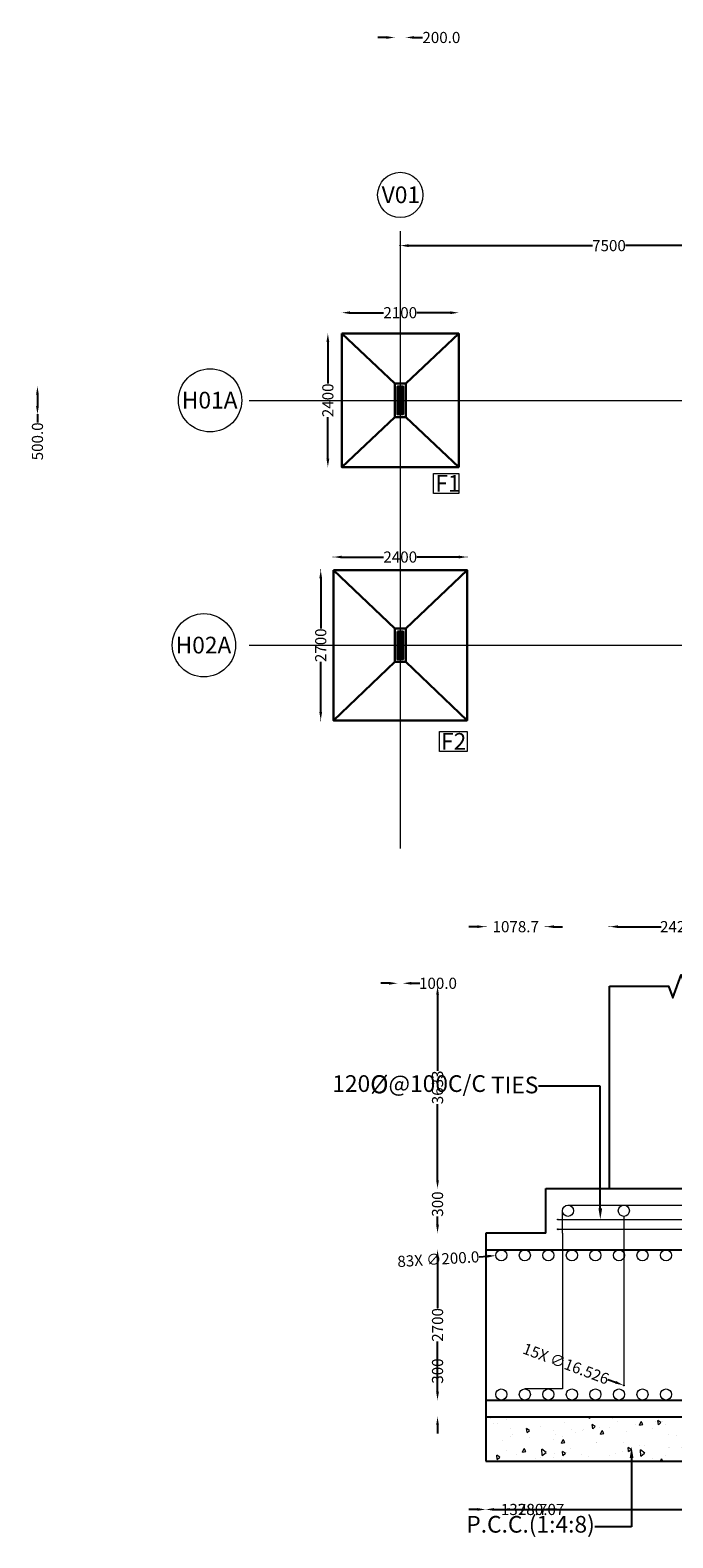
# Model space of a CAD drawing. Units: millimetres. Extents: x -30630 to 20484, y 3580 to 30715.
# Tile 1 of 4: x -30630 to -19082, y 3631 to 30715. Entities that reach past the tile are written whole.
import ezdxf
from ezdxf import colors
from ezdxf.entities.mleader import LeaderData, LeaderLine
from ezdxf.math import Vec2, Vec3

# ---------------------------------------------------------------- set-up
doc = ezdxf.new("R2010")
doc.units = ezdxf.units.MM
doc.header["$MEASUREMENT"] = 0
for name, color, linetype, lineweight in [('S-ANNO-DIMS', 2, 'Continuous', 18), ('S-ANNO-SYMB', 3, 'Continuous', 18), ('S-ANNO-TEXT', 7, 'Continuous', 18), ('S-CONC', 7, 'Continuous', 25), ('S-FNDN', 7, 'Continuous', 30), ('S-FNDN-PATT', 8, 'Continuous', 13), ('S-GRID', 1, 'Continuous', 18), ('S-GRID-IDEN', 7, 'Continuous', 18), ('S-REIN', 1, 'Continuous', 18)]:
    doc.layers.add(name, color=color, linetype=linetype, lineweight=lineweight)
doc.styles.get("Standard").update_dxf_attribs({"font": 'arial.ttf'})
doc.dimstyles.get("Standard").update_dxf_attribs({"dimtxt": 200, "dimasz": 150, "dimexe": 0.18, "dimexo": 0.0625, "dimgap": 0.09, "dimtad": 0, "dimdec": 0, "dimzin": 0, "dimdsep": 46, "dimtxsty": 'Standard', "dimcen": 0.09, "dimadec": 0, "dimazin": 0, "dimtfac": 1, "dimtdec": 0, "dimtofl": 0, "dimtmove": 0, "dimatfit": 3, "dimfxl": 1, "dimfxlon": 1, "dimtolj": 1, "dimtzin": 0, "dimarcsym": 0})

# ---------------------------------------------------------------- blocks, each defined once
blk = doc.blocks.new('*D1')
at = {"layer": 'Defpoints', "color": 0, "transparency": 16777216}
for p in [(-16480, 26844), (-23980, 25951), (-16480, 25951)]:
    blk.add_point(p, dxfattribs=at)
at = {"layer": 'S-ANNO-DIMS', "color": 0, "lineweight": -2, "transparency": 16777216}
for p, q in [((-23980, 26843), (-23980, 26844)), ((-23830, 26844), (-20528, 26844)), ((-16630, 26844), (-19933, 26844)), ((-16480, 26843), (-16480, 26844))]:
    blk.add_line(p, q, dxfattribs=at)
at = {"layer": 'S-ANNO-DIMS', "color": 0, "transparency": 16777216}
for points in [[(-23830, 26869), (-23830, 26819), (-23980, 26844)], [(-16630, 26869), (-16630, 26819), (-16480, 26844)]]:
    blk.add_solid(points, dxfattribs=at)
at = {"layer": 'S-ANNO-DIMS', "color": 0, "transparency": 16777216, "insert": (-20230, 26844), "char_height": 200, "attachment_point": 5}
blk.add_mtext('\\A1;7500', dxfattribs=at)
blk = doc.blocks.new('*D8')
at = {"layer": 'Defpoints', "color": 0, "transparency": 16777216}
for p in [(-22930, 25639), (-25030, 25265), (-22930, 25265)]:
    blk.add_point(p, dxfattribs=at)
at = {"layer": 'S-ANNO-DIMS', "color": 0, "lineweight": -2, "transparency": 16777216}
for p, q in [((-25030, 25638), (-25030, 25639)), ((-24880, 25639), (-24280, 25639)), ((-23080, 25639), (-23680, 25639)), ((-22930, 25638), (-22930, 25639))]:
    blk.add_line(p, q, dxfattribs=at)
at = {"layer": 'S-ANNO-DIMS', "color": 0, "transparency": 16777216}
for points in [[(-24880, 25664), (-24880, 25614), (-25030, 25639)], [(-23080, 25664), (-23080, 25614), (-22930, 25639)]]:
    blk.add_solid(points, dxfattribs=at)
at = {"layer": 'S-ANNO-DIMS', "color": 0, "transparency": 16777216, "insert": (-23980, 25639), "char_height": 200, "attachment_point": 5}
blk.add_mtext('\\A1;2100', dxfattribs=at)
blk = doc.blocks.new('*D9')
at = {"layer": 'Defpoints', "color": 0, "transparency": 16777216}
for p in [(-25030, 25265), (-25281, 22865), (-25030, 22865)]:
    blk.add_point(p, dxfattribs=at)
at = {"layer": 'S-ANNO-DIMS', "color": 0, "lineweight": -2, "transparency": 16777216}
for p, q in [((-25280, 25265), (-25281, 25265)), ((-25281, 25115), (-25281, 24365)), ((-25281, 23015), (-25281, 23765)), ((-25280, 22865), (-25281, 22865))]:
    blk.add_line(p, q, dxfattribs=at)
at = {"layer": 'S-ANNO-DIMS', "color": 0, "transparency": 16777216}
for points in [[(-25306, 25115), (-25256, 25115), (-25281, 25265)], [(-25306, 23015), (-25256, 23015), (-25281, 22865)]]:
    blk.add_solid(points, dxfattribs=at)
at = {"layer": 'S-ANNO-DIMS', "color": 0, "transparency": 16777216, "insert": (-25281, 24065), "char_height": 200, "attachment_point": 5, "rotation": 90}
blk.add_mtext('\\A1;2400', dxfattribs=at)
blk = doc.blocks.new('*D20')
at = {"layer": 'Defpoints', "color": 0, "transparency": 16777216}
for p in [(-25180, 21250), (-25180, 21015), (-22780, 21015)]:
    blk.add_point(p, dxfattribs=at)
at = {"layer": 'S-ANNO-DIMS', "color": 0, "lineweight": -2, "transparency": 16777216}
for p, q in [((-25180, 21249), (-25180, 21251)), ((-25030, 21250), (-24280, 21250)), ((-22930, 21250), (-23680, 21250)), ((-22780, 21249), (-22780, 21251))]:
    blk.add_line(p, q, dxfattribs=at)
at = {"layer": 'S-ANNO-DIMS', "color": 0, "transparency": 16777216}
for points in [[(-25030, 21275), (-25030, 21225), (-25180, 21250)], [(-22930, 21275), (-22930, 21225), (-22780, 21250)]]:
    blk.add_solid(points, dxfattribs=at)
at = {"layer": 'S-ANNO-DIMS', "color": 0, "transparency": 16777216, "insert": (-23980, 21250), "char_height": 200, "attachment_point": 5}
blk.add_mtext('\\A1;2400', dxfattribs=at)
blk = doc.blocks.new('*D21')
at = {"layer": 'Defpoints', "color": 0, "transparency": 16777216}
for p in [(-25180, 21015), (-25409, 18315), (-25180, 18315)]:
    blk.add_point(p, dxfattribs=at)
at = {"layer": 'S-ANNO-DIMS', "color": 0, "lineweight": -2, "transparency": 16777216}
for p, q in [((-25408, 21015), (-25410, 21015)), ((-25409, 20865), (-25409, 19965)), ((-25409, 18465), (-25409, 19365)), ((-25408, 18315), (-25410, 18315))]:
    blk.add_line(p, q, dxfattribs=at)
at = {"layer": 'S-ANNO-DIMS', "color": 0, "transparency": 16777216}
for points in [[(-25434, 20865), (-25384, 20865), (-25409, 21015)], [(-25434, 18465), (-25384, 18465), (-25409, 18315)]]:
    blk.add_solid(points, dxfattribs=at)
at = {"layer": 'S-ANNO-DIMS', "color": 0, "transparency": 16777216, "insert": (-25409, 19665), "char_height": 200, "attachment_point": 5, "rotation": 90}
blk.add_mtext('\\A1;2700', dxfattribs=at)
blk = doc.blocks.new('FOOTING-F1')
h = blk.add_hatch()
h.set_pattern_fill('ANSI31', color=256, scale=100)
h.set_pattern_definition([(45, (50626.339, 2179.544), (-8.8388348, 8.8388348), [])])
h.paths.add_polyline_path([(1100, 24315), (1000, 24315), (1000, 23815), (1100, 23815)])
for p, q in [((0, 25265), (950, 24365)), ((1150, 24365), (2100, 25265)), ((950, 23765), (0, 22865)), ((1150, 23765), (2100, 22865))]:
    blk.add_line(p, q)
for points in [[(0, 25265), (2100, 25265), (2100, 22865), (0, 22865)], [(950, 24365), (1150, 24365), (1150, 23765), (950, 23765)], [(1000, 24315), (1100, 24315), (1100, 23815), (1000, 23815)]]:
    blk.add_lwpolyline(points, close=True)
blk = doc.blocks.new('FOOTING-F2')
h = blk.add_hatch()
h.set_pattern_fill('ANSI31', color=256, scale=100)
h.set_pattern_definition([(45, (58801.161, 2265.705), (-8.8388348, 8.8388348), [])])
h.paths.add_polyline_path([(1250, 19915), (1150, 19915), (1150, 19415), (1250, 19415)])
for p, q in [((1100, 19965), (0, 21015)), ((1300, 19965), (2400, 21015)), ((1100, 19365), (0, 18315)), ((1300, 19365), (2400, 18315))]:
    blk.add_line(p, q)
for points in [[(0, 21015), (2400, 21015), (2400, 18315), (0, 18315)], [(1100, 19965), (1300, 19965), (1300, 19365), (1100, 19365)], [(1150, 19915), (1250, 19915), (1250, 19415), (1150, 19415)]]:
    blk.add_lwpolyline(points, close=True)
blk = doc.blocks.new('*D37')
at = {"layer": 'Defpoints', "color": 0, "transparency": 16777216}
for p in [(-23310, 6106), (-22445, 6106), (-22445, 5806)]:
    blk.add_point(p, dxfattribs=at)
at = {"layer": 'S-ANNO-DIMS', "color": 0, "lineweight": -2, "transparency": 16777216}
for p, q in [((-23310, 6256), (-23310, 6406)), ((-23309, 6106), (-23310, 6106)), ((-23309, 5806), (-23310, 5806)), ((-23310, 5656), (-23310, 5506))]:
    blk.add_line(p, q, dxfattribs=at)
at = {"layer": 'S-ANNO-DIMS', "color": 0, "transparency": 16777216}
for points in [[(-23335, 6256), (-23285, 6256), (-23310, 6106)], [(-23335, 5656), (-23285, 5656), (-23310, 5806)]]:
    blk.add_solid(points, dxfattribs=at)
at = {"layer": 'S-ANNO-DIMS', "color": 0, "transparency": 16777216, "insert": (-23310, 6627), "char_height": 200, "attachment_point": 5, "rotation": 90}
blk.add_mtext('\\A1;300', dxfattribs=at)
blk = doc.blocks.new('*D38')
at = {"layer": 'Defpoints', "color": 0, "transparency": 16777216}
for p in [(-23309.743439, 8806.371523), (-22444.743439, 8806.371523), (-22444.743439, 6106.371523)]:
    blk.add_point(p, dxfattribs=at)
at = {"layer": 'S-ANNO-DIMS', "color": 0, "lineweight": -2, "transparency": 16777216}
for p, q in [((-23308.743439, 8806.371523), (-23309.923439, 8806.371523)), ((-23309.743439, 8656.371523), (-23309.743439, 7756.461523)), ((-23309.743439, 6256.371523), (-23309.743439, 7156.281523)), ((-23308.743439, 6106.371523), (-23309.923439, 6106.371523))]:
    blk.add_line(p, q, dxfattribs=at)
at = {"layer": 'S-ANNO-DIMS', "color": 0, "transparency": 16777216}
for points in [[(-23334.743439, 8656.371523), (-23284.743439, 8656.371523), (-23309.743439, 8806.371523)], [(-23334.743439, 6256.371523), (-23284.743439, 6256.371523), (-23309.743439, 6106.371523)]]:
    blk.add_solid(points, dxfattribs=at)
at = {"layer": 'S-ANNO-DIMS', "color": 0, "transparency": 16777216, "insert": (-23309.743439, 7456.371523), "char_height": 200, "attachment_point": 5, "rotation": 90}
blk.add_mtext('\\A1;2700', dxfattribs=at)
blk = doc.blocks.new('*D39')
at = {"layer": 'Defpoints', "color": 0, "transparency": 16777216}
for p in [(-23310, 9106), (-22445, 9106), (-22445, 8806)]:
    blk.add_point(p, dxfattribs=at)
at = {"layer": 'S-ANNO-DIMS', "color": 0, "lineweight": -2, "transparency": 16777216}
for p, q in [((-23310, 9256), (-23310, 9406)), ((-23309, 9106), (-23310, 9106)), ((-23309, 8806), (-23310, 8806)), ((-23310, 8656), (-23310, 8506))]:
    blk.add_line(p, q, dxfattribs=at)
at = {"layer": 'S-ANNO-DIMS', "color": 0, "transparency": 16777216}
for points in [[(-23335, 9256), (-23285, 9256), (-23310, 9106)], [(-23335, 8656), (-23285, 8656), (-23310, 8806)]]:
    blk.add_solid(points, dxfattribs=at)
at = {"layer": 'S-ANNO-DIMS', "color": 0, "transparency": 16777216, "insert": (-23310, 9627), "char_height": 200, "attachment_point": 5, "rotation": 90}
blk.add_mtext('\\A1;300', dxfattribs=at)
blk = doc.blocks.new('*D40')
at = {"layer": 'Defpoints', "color": 0, "transparency": 16777216}
for p in [(-23310, 13539), (-12091, 13539), (-12091, 9906)]:
    blk.add_point(p, dxfattribs=at)
at = {"layer": 'S-ANNO-DIMS', "color": 0, "lineweight": -2, "transparency": 16777216}
for p, q in [((-23309, 13539), (-23310, 13539)), ((-23310, 13389), (-23310, 12021)), ((-23310, 10056), (-23310, 11424)), ((-23309, 9906), (-23310, 9906))]:
    blk.add_line(p, q, dxfattribs=at)
at = {"layer": 'S-ANNO-DIMS', "color": 0, "transparency": 16777216}
for points in [[(-23335, 13389), (-23285, 13389), (-23310, 13539)], [(-23335, 10056), (-23285, 10056), (-23310, 9906)]]:
    blk.add_solid(points, dxfattribs=at)
at = {"layer": 'S-ANNO-DIMS', "color": 0, "transparency": 16777216, "insert": (-23310, 11723), "char_height": 200, "attachment_point": 5, "rotation": 90}
blk.add_mtext('\\A1;3633', dxfattribs=at)
blk = doc.blocks.new('*D41')
at = {"layer": 'Defpoints', "color": 0, "transparency": 16777216}
for p in [(-21366, 14610), (-22445, 9106), (-21366, 9106)]:
    blk.add_point(p, dxfattribs=at)
at = {"layer": 'S-ANNO-DIMS', "color": 0, "lineweight": -2, "transparency": 16777216}
for p, q in [((-22595, 14610), (-22745, 14610)), ((-22445, 14609), (-22445, 14611)), ((-21366, 14609), (-21366, 14611)), ((-21216, 14610), (-21066, 14610))]:
    blk.add_line(p, q, dxfattribs=at)
at = {"layer": 'S-ANNO-DIMS', "color": 0, "transparency": 16777216}
for points in [[(-22595, 14635), (-22595, 14585), (-22445, 14610)], [(-21216, 14635), (-21216, 14585), (-21366, 14610)]]:
    blk.add_solid(points, dxfattribs=at)
at = {"layer": 'S-ANNO-DIMS', "color": 0, "transparency": 16777216, "insert": (-21905, 14610), "char_height": 200, "attachment_point": 5}
blk.add_mtext('\\A1;1078.7', dxfattribs=at)
blk = doc.blocks.new('*D43')
at = {"layer": 'Defpoints', "color": 0, "transparency": 16777216}
for p in [(-17798, 14610), (-20219, 13539), (-17798, 13539)]:
    blk.add_point(p, dxfattribs=at)
at = {"layer": 'S-ANNO-DIMS', "color": 0, "lineweight": -2, "transparency": 16777216}
for p, q in [((-20219, 14609), (-20219, 14611)), ((-20069, 14610), (-19290, 14610)), ((-17948, 14610), (-18727, 14610)), ((-17798, 14609), (-17798, 14611))]:
    blk.add_line(p, q, dxfattribs=at)
at = {"layer": 'S-ANNO-DIMS', "color": 0, "transparency": 16777216}
for points in [[(-20069, 14635), (-20069, 14585), (-20219, 14610)], [(-17948, 14635), (-17948, 14585), (-17798, 14610)]]:
    blk.add_solid(points, dxfattribs=at)
at = {"layer": 'S-ANNO-DIMS', "color": 0, "transparency": 16777216, "insert": (-19009, 14610), "char_height": 200, "attachment_point": 5}
blk.add_mtext('\\A1;2421', dxfattribs=at)
blk = doc.blocks.new('*D61')
at = {"layer": 'Defpoints', "color": 0, "transparency": 16777216}
for p in [(-19970, 6373), (-19955, 6368)]:
    blk.add_point(p, dxfattribs=at)
at = {"layer": 'S-ANNO-DIMS', "color": 0, "lineweight": -2, "transparency": 16777216}
for p, q in [((-20251, 6478), (-20111, 6426)), ((-19963, 6370), (-19963, 6371)), ((-19963, 6370), (-19962, 6370))]:
    blk.add_line(p, q, dxfattribs=at)
at = {"layer": 'S-ANNO-DIMS', "color": 0, "transparency": 16777216}
blk.add_solid([(-20102, 6449), (-20120, 6402), (-19970, 6373)], dxfattribs=at)
at = {"layer": 'S-ANNO-DIMS', "color": 0, "transparency": 16777216, "insert": (-21002, 6759), "char_height": 200, "attachment_point": 5, "rotation": 339.5143}
blk.add_mtext('\\A1;15X ∅16.526', dxfattribs=at)
blk = doc.blocks.new('*D64')
at = {"layer": 'Defpoints', "color": 0, "transparency": 16777216}
for p in [(-23880, 30583), (-24080, 24365), (-23880, 24365)]:
    blk.add_point(p, dxfattribs=at)
at = {"layer": 'S-ANNO-DIMS', "color": 0, "lineweight": -2, "transparency": 16777216}
for p, q in [((-24230, 30583), (-24380, 30583)), ((-24080, 30582), (-24080, 30584)), ((-23880, 30582), (-23880, 30584)), ((-23730, 30583), (-23580, 30583))]:
    blk.add_line(p, q, dxfattribs=at)
at = {"layer": 'S-ANNO-DIMS', "color": 0, "transparency": 16777216}
for points in [[(-24230, 30608), (-24230, 30558), (-24080, 30583)], [(-23730, 30608), (-23730, 30558), (-23880, 30583)]]:
    blk.add_solid(points, dxfattribs=at)
at = {"layer": 'S-ANNO-DIMS', "color": 0, "transparency": 16777216, "insert": (-23241, 30583), "char_height": 200, "attachment_point": 5}
blk.add_mtext('\\A1;200.0', dxfattribs=at)
blk = doc.blocks.new('*D65')
at = {"layer": 'Defpoints', "color": 0, "transparency": 16777216}
for p in [(-23880, 24365), (-23880, 23765), (19772, 23765)]:
    blk.add_point(p, dxfattribs=at)
at = {"layer": 'S-ANNO-DIMS', "color": 0, "lineweight": -2, "transparency": 16777216}
for p, q in [((19771, 24365), (19772, 24365)), ((19772, 24215), (19772, 23915)), ((19771, 23765), (19772, 23765)), ((19772, 23765), (19772, 23615))]:
    blk.add_line(p, q, dxfattribs=at)
at = {"layer": 'S-ANNO-DIMS', "color": 0, "transparency": 16777216}
for points in [[(19747, 24215), (19797, 24215), (19772, 24365)], [(19747, 23915), (19797, 23915), (19772, 23765)]]:
    blk.add_solid(points, dxfattribs=at)
at = {"layer": 'S-ANNO-DIMS', "color": 0, "transparency": 16777216, "insert": (19772, 23277), "char_height": 200, "attachment_point": 5, "rotation": 90}
blk.add_mtext('\\A1;600.0', dxfattribs=at)
blk = doc.blocks.new('*D66')
at = {"layer": 'Defpoints', "color": 0, "transparency": 16777216}
for p in [(-24030, 23815), (-23930, 23815), (-23930, 13593)]:
    blk.add_point(p, dxfattribs=at)
at = {"layer": 'S-ANNO-DIMS', "color": 0, "lineweight": -2, "transparency": 16777216}
for p, q in [((-24180, 13593), (-24330, 13593)), ((-24030, 13594), (-24030, 13593)), ((-23930, 13594), (-23930, 13593)), ((-23780, 13593), (-23630, 13593))]:
    blk.add_line(p, q, dxfattribs=at)
at = {"layer": 'S-ANNO-DIMS', "color": 0, "transparency": 16777216}
for points in [[(-24180, 13618), (-24180, 13568), (-24030, 13593)], [(-23780, 13618), (-23780, 13568), (-23930, 13593)]]:
    blk.add_solid(points, dxfattribs=at)
at = {"layer": 'S-ANNO-DIMS', "color": 0, "transparency": 16777216, "insert": (-23302, 13593), "char_height": 200, "attachment_point": 5}
blk.add_mtext('\\A1;100.0', dxfattribs=at)
blk = doc.blocks.new('*D67')
at = {"layer": 'Defpoints', "color": 0, "transparency": 16777216}
for p in [(-24030, 24315), (-30499, 23815), (-24030, 23815)]:
    blk.add_point(p, dxfattribs=at)
at = {"layer": 'S-ANNO-DIMS', "color": 0, "lineweight": -2, "transparency": 16777216}
for p, q in [((-30498, 24315), (-30499, 24315)), ((-30499, 24165), (-30499, 23965)), ((-30498, 23815), (-30499, 23815)), ((-30499, 23815), (-30499, 23665))]:
    blk.add_line(p, q, dxfattribs=at)
at = {"layer": 'S-ANNO-DIMS', "color": 0, "transparency": 16777216}
for points in [[(-30524, 24165), (-30474, 24165), (-30499, 24315)], [(-30524, 23965), (-30474, 23965), (-30499, 23815)]]:
    blk.add_solid(points, dxfattribs=at)
at = {"layer": 'S-ANNO-DIMS', "color": 0, "transparency": 16777216, "insert": (-30499, 23328), "char_height": 200, "attachment_point": 5, "rotation": 90}
blk.add_mtext('\\A1;500.0', dxfattribs=at)
blk = doc.blocks.new('*D68')
at = {"layer": 'Defpoints', "color": 0, "transparency": 16777216}
for p in [(-22445, 6106), (-7445, 6106), (-7445, 4141)]:
    blk.add_point(p, dxfattribs=at)
at = {"layer": 'S-ANNO-DIMS', "color": 0, "lineweight": -2, "transparency": 16777216}
for p, q in [((-22445, 4142), (-22445, 4141)), ((-22295, 4141), (-15428, 4141)), ((-7595, 4141), (-14462, 4141)), ((-7445, 4142), (-7445, 4141))]:
    blk.add_line(p, q, dxfattribs=at)
at = {"layer": 'S-ANNO-DIMS', "color": 0, "transparency": 16777216}
for points in [[(-22295, 4166), (-22295, 4116), (-22445, 4141)], [(-7595, 4166), (-7595, 4116), (-7445, 4141)]]:
    blk.add_solid(points, dxfattribs=at)
at = {"layer": 'S-ANNO-DIMS', "color": 0, "transparency": 16777216, "insert": (-14945, 4141), "char_height": 200, "attachment_point": 5}
blk.add_mtext('\\A1;15000.0', dxfattribs=at)
blk = doc.blocks.new('*D69')
at = {"layer": 'Defpoints', "color": 0, "transparency": 16777216}
for p in [(-22445, 6106), (-22165, 6206), (-22165, 4141)]:
    blk.add_point(p, dxfattribs=at)
at = {"layer": 'S-ANNO-DIMS', "color": 0, "lineweight": -2, "transparency": 16777216}
for p, q in [((-22595, 4141), (-22745, 4141)), ((-22445, 4142), (-22445, 4141)), ((-22165, 4142), (-22165, 4141)), ((-22015, 4141), (-21865, 4141))]:
    blk.add_line(p, q, dxfattribs=at)
at = {"layer": 'S-ANNO-DIMS', "color": 0, "transparency": 16777216}
for points in [[(-22595, 4166), (-22595, 4116), (-22445, 4141)], [(-22015, 4166), (-22015, 4116), (-22165, 4141)]]:
    blk.add_solid(points, dxfattribs=at)
at = {"layer": 'S-ANNO-DIMS', "color": 0, "transparency": 16777216, "insert": (-21448, 4141), "char_height": 200, "attachment_point": 5}
blk.add_mtext('\\A1;280.07', dxfattribs=at)
blk = doc.blocks.new('*D71')
at = {"layer": 'Defpoints', "color": 0, "transparency": 16777216}
for p in [(-21066, 6306), (-22445, 6106), (-21066, 4141)]:
    blk.add_point(p, dxfattribs=at)
at = {"layer": 'S-ANNO-DIMS', "color": 0, "lineweight": -2, "transparency": 16777216}
for p, q in [((-22445, 4142), (-22445, 4141)), ((-22295, 4141), (-22161, 4141)), ((-21216, 4141), (-21350, 4141)), ((-21066, 4142), (-21066, 4141))]:
    blk.add_line(p, q, dxfattribs=at)
at = {"layer": 'S-ANNO-DIMS', "color": 0, "transparency": 16777216}
for points in [[(-22295, 4166), (-22295, 4116), (-22445, 4141)], [(-21216, 4166), (-21216, 4116), (-21066, 4141)]]:
    blk.add_solid(points, dxfattribs=at)
at = {"layer": 'S-ANNO-DIMS', "color": 0, "transparency": 16777216, "insert": (-21755, 4141), "char_height": 200, "attachment_point": 5}
blk.add_mtext('\\A1;1378.7', dxfattribs=at)
blk = doc.blocks.new('*D80')
at = {"layer": 'Defpoints', "color": 0, "transparency": 16777216}
for p in [(-22264, 8700), (-22065, 8712)]:
    blk.add_point(p, dxfattribs=at)
at = {"layer": 'S-ANNO-DIMS', "color": 0, "lineweight": -2, "transparency": 16777216}
for p, q in [((-22564, 8682), (-22414, 8691)), ((-22165, 8706), (-22165, 8706)), ((-22165, 8706), (-22165, 8706))]:
    blk.add_line(p, q, dxfattribs=at)
at = {"layer": 'S-ANNO-DIMS', "color": 0, "transparency": 16777216}
blk.add_solid([(-22416, 8716), (-22413, 8666), (-22264, 8700)], dxfattribs=at)
at = {"layer": 'S-ANNO-DIMS', "color": 0, "transparency": 16777216, "insert": (-23296, 8638), "char_height": 200, "attachment_point": 5, "rotation": 3.4778}
blk.add_mtext('\\A1;83X ∅200.0', dxfattribs=at)

msp = doc.modelspace()

# ---------------------------------------------------------------- hatches: boundary and pattern name
at = {"layer": 'S-FNDN-PATT'}
h = msp.add_hatch(dxfattribs=at)
h.set_pattern_fill('AR-CONC', color=256, scale=100, angle=47)
h.set_pattern_definition([(97, (-6254.7, 5540.77), (535.064, 481.774), [75, -825]), (42, (-6254.7, 5540.8), (-644.747, 411.518), [60, -660]), (147.4514, (-6210.1, 5580.9), (-109.682, 893.292), [63.74, -701.142]), (93.184, (-6401, 5677.2), (848.91, 667.647), [112.5, -1237.5]), (143.636, (-6330.2, 5732.8), (-74.99, 1347.916), [95.61, -1051.714]), (38.184, (-6401, 5677.2), (-74.99, 1347.916), [90, -990]), (68, (-6296.2, 5716.2), (701.546, 161.965), [75, -825]), (13, (-6296.2, 5716.2), (-364.4, 672.5), [60, -660]), (118.4514, (-6237.74, 5729.7), (337.146, 834.465), [63.74, -701.142]), (84.5, (-6254.7, 5540.77), (-235.17, 235.9262), [0, -652, 0, -670, 0, -662.5]), (54.5, (-6254.7, 5540.77), (-109.0415, 461.385), [0, -382, 0, -637, 0, -252.5]), (14.5, (-6406.8, 5377.67), (380.5616, 375.0306), [0, -250, 0, -780, 0, -1035]), (4.5, (-6475, 5304.54), (324.52, 494.787), [0, -325, 0, -518, 0, -735])])
h.paths.add_polyline_path([(-7444.7434, 5006.3715), (-7444.7434, 5806.3715), (-22444.7434, 5806.3715), (-22444.7434, 5006.3715)])

# ---------------------------------------------------------------- linework, layer by layer
at = {"layer": 'S-ANNO-SYMB'}
for points in [[(-23380.1095, 22391.7904), (-23380.1095, 22753.0183), (-22930.0685, 22753.0183), (-22930.0685, 22391.7904)], [(-23277.1763, 17757.175), (-23277.1763, 18118.4029), (-22780.0685, 18118.4029), (-22780.0685, 17757.175)]]:
    msp.add_lwpolyline(points, close=True, dxfattribs=at)
at = {"layer": 'S-CONC'}
for p, q in [((-20219.1563, 9906.3715), (-20219.1563, 13539.302)), ((-21366.0811, 9106.3715), (-21366.0811, 9906.3715)), ((-21366.0811, 9906.3715), (-14944.7434, 9906.3715)), ((-22444.7434, 9106.3715), (-22444.7434, 5806.3715)), ((-21366.0811, 9106.3715), (-22444.7434, 9106.3715)), ((-22444.7434, 8806.3715), (-7444.7434, 8806.3715)), ((-22444.7434, 6106.3715), (-7444.7434, 6106.3715)), ((-22444.7434, 5806.3715), (-7444.7434, 5806.3715)), ((-22444.7434, 5806.3715), (-22444.7434, 5006.3715)), ((-22444.7434, 5006.3715), (-7444.7434, 5006.3715))]:
    msp.add_line(p, q, dxfattribs=at)
msp.add_lwpolyline([(-20219.3363, 13539.302), (-19158.6753, 13539.302), (-19083.6753, 13333.2412), (-18933.6753, 13745.3628), (-18858.6753, 13539.302), (-17798.0143, 13539.302)], dxfattribs=at)
at = {"layer": 'S-GRID'}
for p, q in [((-23980.0685, 27102.0571), (-23980.0685, 16015.6561)), ((-26695.8159, 24064.7195), (17349.3354, 24064.7195)), ((-26695.8159, 19664.7195), (17349.3354, 19664.7195))]:
    msp.add_line(p, q, dxfattribs=at)
at = {"layer": 'S-GRID-IDEN'}
for centre, radius in [((-23980.0685, 27753.8802), 407.0061), ((-27396.6824, 24064.7195), 568.051), ((-27508.1703, 19664.7195), 568.051)]:
    msp.add_circle(centre, radius, dxfattribs=at)
at = {"layer": 'S-REIN'}
for p, q in [((-21066.0811, 9106.3715), (-21066.0811, 9506.3715)), ((-20966.0811, 9606.3715), (-14944.7434, 9606.3715)), ((-21140.5094, 9349.192), (-8740.6319, 9349.192)), ((-19962.5248, 9406.3715), (-19962.5248, 6378.7119)), ((-21140.5094, 9174.6041), (-8740.6319, 9174.6041)), ((-21066.0811, 9106.3715), (-21066.0811, 6306.3715)), ((-21066.0811, 6306.3715), (-21741.8353, 6306.3715))]:
    msp.add_line(p, q, dxfattribs=at)
for centre, radius in [((-20966.0811, 9506.3715), 100), ((-19962.5248, 9506.3715), 100), ((-21148.7724, 9349.192), 8.263), ((-21148.7724, 9174.6041), 8.263), ((-22164.6749, 8706.3715), 100), ((-21741.8353, 8706.3715), 100), ((-21318.9956, 8706.3715), 100), ((-20896.1559, 8706.3715), 100), ((-20473.3162, 8706.3715), 100), ((-20050.4765, 8706.3715), 100), ((-19627.6368, 8706.3715), 100), ((-19204.7972, 8706.3715), 100), ((-22164.6749, 6206.3715), 100), ((-21741.8353, 6206.3715), 100), ((-21318.9956, 6206.3715), 100), ((-20896.1559, 6206.3715), 100), ((-20473.3162, 6206.3715), 100), ((-20050.4765, 6206.3715), 100), ((-19962.5248, 6370.4489), 8.263), ((-19627.6368, 6206.3715), 100), ((-19204.7972, 6206.3715), 100)]:
    msp.add_circle(centre, radius, dxfattribs=at)

# ---------------------------------------------------------------- block references
at = {"layer": 'S-FNDN'}
for name, p in [('FOOTING-F1', (-25030.069, 0)), ('FOOTING-F2', (-25180.069, 0))]:
    msp.add_blockref(name, p, dxfattribs=at)

# ---------------------------------------------------------------- texts
at = {"layer": 'S-ANNO-TEXT', "char_height": 300, "attachment_point": 1}
for s, width, insert in [('V01', 4876.019723, (-24313.5269, 27907.0521)), ('H01A', 4876.019723, (-27904.3905, 24217.8914)), ('{\\fArial|b1|i0|c0|p34;F1}', 1058.385802, (-23350.1095, 22723.0183)), ('H02A', 4876.019723, (-28015.8784, 19817.8914)), ('{\\fArial|b1|i0|c0|p34;F2}', 1058.385802, (-23247.1763, 18088.4029))]:
    msp.add_mtext_dynamic_manual_height_columns(s, width=width, gutter_width=1, heights=[0], dxfattribs=dict(at, insert=insert))

# ---------------------------------------------------------------- dimensions: what is measured, and where the dimension line sits
at = {"layer": 'S-ANNO-DIMS'}
for base, p1, p2, override, picture, middle in [((-23880.0685, 30583.3863), (-24080.0685, 24364.7195), (-23880.0685, 24364.7195), {"dimdec": 1, "dimlfac": 1, "dimrnd": 0, "dimzin": 0, "dimdsep": 46, "dimlunit": 2}, '*D64', (-23241.1654, 30583.3863)), ((-16480.0685, 26843.6702), (-23980.0685, 25950.8365), (-16480.0685, 25950.8365), {"dimclrd": 0, "dimclre": 0, "dimclrt": 0}, '*D1', (-20230.0685, 26843.6702)), ((-22930.0685, 25638.5997), (-25030.0685, 25264.7195), (-22930.0685, 25264.7195), {"dimclrd": 0, "dimclre": 0, "dimclrt": 0}, '*D8', (-23980.0685, 25638.5997)), ((-23930.0685, 13593.1561), (-24030.0685, 23814.7195), (-23930.0685, 23814.7195), {"dimdec": 1, "dimlfac": 1, "dimrnd": 0, "dimzin": 0, "dimdsep": 46, "dimlunit": 2}, '*D66', (-23302.2841, 13593.1561)), ((-25180.0685, 21250.447), (-22780.0685, 21014.7195), (-25180.0685, 21014.7195), {"dimclrd": 0, "dimclre": 0, "dimclrt": 0}, '*D20', (-23980.0685, 21250.447)), ((-21366.0811, 14610.3628), (-22444.7434, 9106.3715), (-21366.0811, 9106.3715), {"dimdec": 1, "dimlfac": 1, "dimrnd": 0, "dimzin": 0, "dimdsep": 46, "dimlunit": 2}, '*D41', (-21905.4123, 14610.3628)), ((-17798.0143, 14610.3628), (-20219.1563, 13539.302), (-17798.0143, 13539.302), {"dimdec": 0, "dimlfac": 1, "dimrnd": 0, "dimzin": 0, "dimdsep": 46, "dimlunit": 2}, '*D43', (-19008.5853, 14610.3628)), ((-21066.0811, 4141.3715), (-22444.7434, 6106.3715), (-21066.0811, 6306.3715), {"dimdec": 1, "dimlfac": 1, "dimrnd": 0, "dimzin": 0, "dimdsep": 46, "dimlunit": 2}, '*D71', (-21755.4123, 4141.3715)), ((-22164.6749, 4141.3715), (-22444.7434, 6106.3715), (-22164.6749, 6206.3715), {"dimdec": 2, "dimlfac": 1, "dimrnd": 0, "dimzin": 0, "dimdsep": 46, "dimlunit": 2}, '*D69', (-21447.7364, 4141.3715)), ((-7444.7434, 4141.3715), (-22444.7434, 6106.3715), (-7444.7434, 6106.3715), {"dimdec": 1, "dimlfac": 1, "dimrnd": 0, "dimzin": 0, "dimdsep": 46, "dimlunit": 2}, '*D68', (-14944.7434, 4141.3715))]:
    dim = msp.add_linear_dim(base=base, p1=p1, p2=p2, dimstyle='Standard', override=override, dxfattribs=at)
    dim.commit()
    dim.dimension.update_dxf_attribs({"geometry": picture, "text_midpoint": middle})
for base, p1, p2, override, picture, middle in [((-25281.1139, 22864.7195), (-25030.0685, 25264.7195), (-25030.0685, 22864.7195), {"dimclrd": 0, "dimclre": 0, "dimclrt": 0}, '*D9', (-25281.1139, 24064.7195)), ((-30498.7213, 23814.7195), (-24030.0685, 24314.7195), (-24030.0685, 23814.7195), {"dimdec": 1, "dimlfac": 1, "dimrnd": 0, "dimzin": 0, "dimdsep": 46, "dimlunit": 2}, '*D67', (-30498.7213, 23327.5217)), ((19771.8354, 23764.7195), (-23880.0685, 24364.7195), (-23880.0685, 23764.7195), {"dimdec": 1, "dimlfac": 1, "dimrnd": 0, "dimzin": 0, "dimdsep": 46, "dimlunit": 2}, '*D65', (19771.8354, 23276.976)), ((-25409.3967, 18314.7195), (-25180.0685, 21014.7195), (-25180.0685, 18314.7195), {"dimclrd": 0, "dimclre": 0, "dimclrt": 0}, '*D21', (-25409.3967, 19664.7195)), ((-23309.7434, 13539.302), (-12091.2926, 9906.3715), (-12091.2926, 13539.302), {"dimdec": 0, "dimlfac": 1, "dimrnd": 0, "dimzin": 0, "dimdsep": 46, "dimlunit": 2}, '*D40', (-23309.7434, 11722.8368)), ((-23309.7434, 9106.3715), (-22444.7434, 8806.3715), (-22444.7434, 9106.3715), {"dimdec": 0, "dimlfac": 1, "dimrnd": 0, "dimzin": 0, "dimdsep": 46, "dimlunit": 2}, '*D39', (-23309.7434, 9626.9936)), ((-23309.7434, 8806.3715), (-22444.7434, 6106.3715), (-22444.7434, 8806.3715), {"dimdec": 0, "dimlfac": 1, "dimrnd": 0, "dimzin": 0, "dimdsep": 46, "dimlunit": 2}, '*D38', (-23309.7434, 7456.3715)), ((-23309.7434, 6106.3715), (-22444.7434, 5806.3715), (-22444.7434, 6106.3715), {"dimdec": 0, "dimlfac": 1, "dimrnd": 0, "dimzin": 0, "dimdsep": 46, "dimlunit": 2}, '*D37', (-23309.7434, 6626.9936))]:
    dim = msp.add_linear_dim(base=base, p1=p1, p2=p2, angle=90, dimstyle='Standard', override=override, dxfattribs=at)
    dim.commit()
    dim.dimension.update_dxf_attribs({"geometry": picture, "text_midpoint": middle})
dim = msp.add_diameter_dim_2p(p1=(-22064.8591, 8712.4377), p2=(-22264.4908, 8700.3053), text='83X <>', dimstyle='Standard', override={"dimdec": 1, "dimlfac": 1, "dimrnd": 0, "dimzin": 0, "dimdsep": 46, "dimlunit": 2}, dxfattribs=at)
dim.commit()
dim.dimension.update_dxf_attribs({"geometry": '*D80', "text_midpoint": (-23295.9655, 8637.6187)})
dim = msp.add_diameter_dim_2p(p1=(-19954.7844, 6367.557), p2=(-19970.2653, 6373.3407), text='15X <>', dimstyle='Standard', override={"dimdec": 3, "dimlfac": 1, "dimrnd": 0, "dimzin": 0, "dimdsep": 46, "dimlunit": 2}, dxfattribs=at)
dim.commit()
dim.dimension.update_dxf_attribs({"geometry": '*D61', "text_midpoint": (-21002.3826, 6758.9398), "dimtype": 163})

# ---------------------------------------------------------------- leaders
at = {"layer": 'S-ANNO-TEXT'}
ml = msp.add_multileader_mtext('Standard', dxfattribs=at)
ml.set_content('120{\\H1.08333x;Ø}@100C/C TIES', color=256)
ml.set_leader_properties()
ml.build(insert=Vec2(0, 0))
ml.multileader.update_dxf_attribs({"dogleg_length": 0.36, "arrow_head_size": 200})
ctx = ml.context
ctx.base_point, ctx.char_height, ctx.arrow_head_size, ctx.landing_gap_size, ctx.plane_origin = Vec3(-25377.4535, 11747.137), 300, 200, 0.09, Vec3(-20385.4241, 9349.192)
ctx.text_align_type = 2
notes = []
notes.append((ctx, [(0, (1, 1, 0), (-21497.6343, 11747.137), (-1, 0), 0.36, [(0, [(-20385.4241, 9349.192), (-20385.4241, 11747.137)], 0, [])])]))
ctx.mtext.insert, ctx.mtext.alignment, ctx.mtext.flow_direction = Vec3(-21498.0843, 11941.2366), 3, 5
ml = msp.add_multileader_mtext('Standard', dxfattribs=at)
ml.set_content('P.C.C.(1:4:8)', color=256)
ml.set_leader_properties()
ml.build(insert=Vec2(0, 0))
ml.multileader.update_dxf_attribs({"dogleg_length": 0.36, "arrow_head_size": 200})
ctx = ml.context
ctx.base_point, ctx.char_height, ctx.arrow_head_size, ctx.landing_gap_size, ctx.plane_origin = Vec3(-22882.6824, 3830.7058), 300, 200, 0.09, Vec3(-19823.6001, 5268.1322)
ctx.text_align_type = 2
notes.append((ctx, [(0, (1, 1, 0), (-20484.1887, 3830.7058), (-1, 0), 0.36, [(0, [(-19823.6001, 5268.1322), (-19823.6001, 3830.7058)], 0, [])])]))
ctx.mtext.insert, ctx.mtext.alignment, ctx.mtext.flow_direction = Vec3(-20484.6387, 4024.8054), 3, 5
for ctx, leaders in notes:
    for number, flags, end, landing, length, lines in leaders:
        leader = LeaderData()
        leader.index, (leader.has_last_leader_line, leader.has_dogleg_vector, leader.attachment_direction) = number, flags
        leader.last_leader_point, leader.dogleg_vector, leader.dogleg_length = Vec3(end), Vec3(landing), length
        for number, points, colour, breaks in lines:
            line = LeaderLine()
            line.index, line.vertices, line.color, line.breaks = number, Vec3.list(points), colors.encode_raw_color(colour), breaks
            leader.lines.append(line)
        ctx.leaders.append(leader)

doc.saveas('drawing.dxf')
